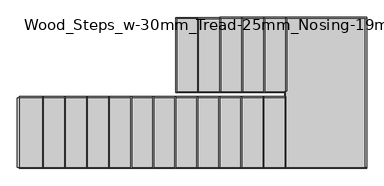
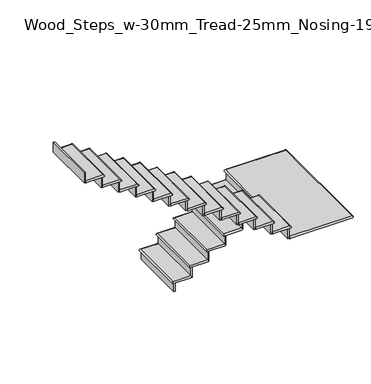
"""IFC4 building model written with IfcOpenShell, lengths in millimetres: stair flight geometry, Wood_Steps_w-30mm_Tread-25mm_Nosing-19mm_Riser."""

from ifc_helpers import new_model, si_unit, frame, origin, place, context, project, spatial, circle_curve, ellipse_curve, faceted_brep, source, transform, mapped, element, save
from ifc_brep_helpers import plane_surface, cylinder_surface, advanced_brep


def wood_steps_w_30mm_tread_25mm_nosing_19mm_riser_5243a390(model_context):
    return source(origin(), model_context, "Body", "SolidModel", [
        advanced_brep(
        [(-8665.149573, -11058.3255223, 782.8), (-8665.149573, -11058.3255223, 812.8), (-8665.149573, -10219.6521308, 812.8), (-8665.149573, -10219.6521308, 782.8), (-8400.9545789, -11058.3255223, 812.8), (-8400.9545789, -10219.6521308, 812.8), (-8400.9545789, -10219.6521308, 782.8), (-8400.9545789, -11058.3255223, 782.8)],
        [
            (0, 1, ellipse_curve(frame((-8665.149573, -11058.3255223, 797.8), z_axis=(-0.707106781186546, 0.707106781186549, 0.0), x_axis=(-0.707106781186549, -0.7071067811865461, 0.0)), 21.2132034, 15.0)),
            (1, 2),
            (2, 3, ellipse_curve(frame((-8665.149573, -10219.6521308, 797.8), z_axis=(-0.7071067811865489, -0.7071067811865461, 0.0), x_axis=(0.7071067811865462, -0.7071067811865489, 0.0)), 21.2132034, 15.0)),
            (3, 0),
            (4, 5),
            (5, 2),
            (1, 4),
            (6, 7),
            (7, 0),
            (3, 6),
            (4, 7, circle_curve(frame((-8400.9545789, -11058.3255223, 797.8), z_axis=(1.0, 0.0, 0.0), x_axis=(0.0, 1.0, 0.0)), 15.0)),
            (6, 5, circle_curve(frame((-8400.9545789, -10219.6521308, 797.8), z_axis=(1.0, 0.0, 0.0), x_axis=(0.0, -1.0, 0.0)), 15.0)),
        ],
        [
            cylinder_surface(frame((-8665.149573, -11058.3255223, 797.8), z_axis=(0.0, -1.0, 0.0), x_axis=(1.0, 0.0, 0.0)), 15.0),
            plane_surface(frame((-6495.4132565, -10219.6521308, 812.8), z_axis=(0.0, 0.0, 1.0), x_axis=(-1.0, 0.0, 0.0))),
            plane_surface(frame((-6495.4132565, -10219.6521308, 782.8), z_axis=(0.0, 0.0, -1.0), x_axis=(1.0, 0.0, 0.0))),
            plane_surface(frame((-8400.9545789, -11058.3255223, 812.8), z_axis=(1.0, 0.0, 0.0), x_axis=(0.0, 0.0, -1.0))),
            cylinder_surface(frame((-8400.9545789, -11058.3255223, 797.8), z_axis=(1.0, 0.0, 0.0), x_axis=(0.0, 1.0, 0.0)), 15.0),
            cylinder_surface(frame((-8665.149573, -10219.6521308, 797.8), z_axis=(-1.0, 0.0, 0.0), x_axis=(0.0, -1.0, 0.0)), 15.0),
        ],
        [
            (0, [[1, 2, 3, 4]]),
            (1, [[5, 6, -2, 7]]),
            (2, [[8, 9, -4, 10]]),
            (3, [[-5, 11, -8, 12]]),
            (4, [[-11, -7, -1, -9]]),
            (5, [[-3, -6, -12, -10]]),
        ],
    ),
        faceted_brep([(-8655.149573, -11058.3255223, 782.8), (-8655.149573, -11058.3255223, 650.24), (-8636.149573, -11058.3255223, 650.24), (-8636.149573, -11058.3255223, 782.8), (-8655.149573, -10219.6521308, 782.8), (-8636.149573, -10219.6521308, 782.8), (-8636.149573, -10219.6521308, 650.24), (-8655.149573, -10219.6521308, 650.24)], [[[0, 1, 2, 3]], [[4, 5, 6, 7]], [[1, 0, 4, 7]], [[2, 1, 7, 6]], [[3, 2, 6, 5]], [[0, 3, 5, 4]]]),
        faceted_brep([(-8400.9545789, -11058.3255223, 945.36), (-8400.9545789, -11058.3255223, 782.8), (-8381.9545789, -11058.3255223, 782.8), (-8381.9545789, -11058.3255223, 945.36), (-8400.9545789, -10219.6521308, 945.36), (-8381.9545789, -10219.6521308, 945.36), (-8381.9545789, -10219.6521308, 782.8), (-8400.9545789, -10219.6521308, 782.8)], [[[0, 1, 2, 3]], [[4, 5, 6, 7]], [[1, 0, 4, 7]], [[2, 1, 7, 6]], [[3, 2, 6, 5]], [[0, 3, 5, 4]]]),
        advanced_brep(
        [(-8146.7595849, -11058.3255223, 975.36), (-8146.7595849, -10219.6521308, 975.36), (-8410.9545789, -10219.6521308, 975.36), (-8410.9545789, -11058.3255223, 975.36), (-8146.7595849, -10219.6521308, 945.36), (-8146.7595849, -11058.3255223, 945.36), (-8410.9545789, -11058.3255223, 945.36), (-8410.9545789, -10219.6521308, 945.36)],
        [
            (0, 1),
            (1, 2),
            (2, 3),
            (3, 0),
            (4, 5),
            (5, 6),
            (6, 7),
            (7, 4),
            (0, 5, circle_curve(frame((-8146.7595849, -11058.3255223, 960.36), z_axis=(1.0, 0.0, 0.0), x_axis=(0.0, 1.0, 0.0)), 15.0)),
            (4, 1, circle_curve(frame((-8146.7595849, -10219.6521308, 960.36), z_axis=(1.0, 0.0, 0.0), x_axis=(0.0, -1.0, 0.0)), 15.0)),
            (6, 3, ellipse_curve(frame((-8410.9545789, -11058.3255223, 960.36), z_axis=(-0.707106781186546, 0.707106781186549, 0.0), x_axis=(-0.707106781186549, -0.7071067811865461, 0.0)), 21.2132034, 15.0)),
            (2, 7, ellipse_curve(frame((-8410.9545789, -10219.6521308, 960.36), z_axis=(-0.7071067811865489, -0.7071067811865461, 0.0), x_axis=(0.7071067811865462, -0.7071067811865489, 0.0)), 21.2132034, 15.0)),
        ],
        [
            plane_surface(frame((-6495.4132565, -10219.6521308, 975.36), z_axis=(0.0, 0.0, 1.0), x_axis=(-1.0, 0.0, 0.0))),
            plane_surface(frame((-6495.4132565, -10219.6521308, 945.36), z_axis=(0.0, 0.0, -1.0), x_axis=(1.0, 0.0, 0.0))),
            plane_surface(frame((-8146.7595849, -11058.3255223, 975.36), z_axis=(1.0, 0.0, 0.0), x_axis=(0.0, 0.0, -1.0))),
            cylinder_surface(frame((-8410.9545789, -11058.3255223, 960.36), z_axis=(0.0, -1.0, 0.0), x_axis=(1.0, 0.0, 0.0)), 15.0),
            cylinder_surface(frame((-8146.7595849, -11058.3255223, 960.36), z_axis=(1.0, 0.0, 0.0), x_axis=(0.0, 1.0, 0.0)), 15.0),
            cylinder_surface(frame((-8410.9545789, -10219.6521308, 960.36), z_axis=(-1.0, 0.0, 0.0), x_axis=(0.0, -1.0, 0.0)), 15.0),
        ],
        [
            (0, [[1, 2, 3, 4]]),
            (1, [[5, 6, 7, 8]]),
            (2, [[-1, 9, -5, 10]]),
            (3, [[11, -3, 12, -7]]),
            (4, [[-9, -4, -11, -6]]),
            (5, [[-12, -2, -10, -8]]),
        ],
    ),
        faceted_brep([(-8146.7595849, -11058.3255223, 1107.92), (-8146.7595849, -11058.3255223, 945.36), (-8127.7595849, -11058.3255223, 945.36), (-8127.7595849, -11058.3255223, 1107.92), (-8146.7595849, -10219.6521308, 1107.92), (-8127.7595849, -10219.6521308, 1107.92), (-8127.7595849, -10219.6521308, 945.36), (-8146.7595849, -10219.6521308, 945.36)], [[[0, 1, 2, 3]], [[4, 5, 6, 7]], [[1, 0, 4, 7]], [[2, 1, 7, 6]], [[3, 2, 6, 5]], [[0, 3, 5, 4]]]),
        advanced_brep(
        [(-7893.1206135, -11058.3255223, 1137.92), (-7893.1206135, -10219.6521308, 1137.92), (-8156.7595849, -10219.6521308, 1137.92), (-8156.7595849, -11058.3255223, 1137.92), (-7893.1206135, -10219.6521308, 1107.92), (-7893.1206135, -11058.3255223, 1107.92), (-8156.7595849, -11058.3255223, 1107.92), (-8156.7595849, -10219.6521308, 1107.92)],
        [
            (0, 1),
            (1, 2),
            (2, 3),
            (3, 0),
            (4, 5),
            (5, 6),
            (6, 7),
            (7, 4),
            (0, 5, circle_curve(frame((-7893.1206135, -11058.3255223, 1122.92), z_axis=(1.0, 0.0, 0.0), x_axis=(0.0, 1.0, 0.0)), 15.0)),
            (4, 1, circle_curve(frame((-7893.1206135, -10219.6521308, 1122.92), z_axis=(1.0, 0.0, 0.0), x_axis=(0.0, -1.0, 0.0)), 15.0)),
            (6, 3, ellipse_curve(frame((-8156.7595849, -11058.3255223, 1122.92), z_axis=(-0.707106781186546, 0.707106781186549, 0.0), x_axis=(-0.707106781186549, -0.7071067811865461, 0.0)), 21.2132034, 15.0)),
            (2, 7, ellipse_curve(frame((-8156.7595849, -10219.6521308, 1122.92), z_axis=(-0.7071067811865489, -0.7071067811865461, 0.0), x_axis=(0.7071067811865462, -0.7071067811865489, 0.0)), 21.2132034, 15.0)),
        ],
        [
            plane_surface(frame((-6495.4132565, -10219.6521308, 1137.92), z_axis=(0.0, 0.0, 1.0), x_axis=(-1.0, 0.0, 0.0))),
            plane_surface(frame((-6495.4132565, -10219.6521308, 1107.92), z_axis=(0.0, 0.0, -1.0), x_axis=(1.0, 0.0, 0.0))),
            plane_surface(frame((-7893.1206135, -11058.3255223, 1137.92), z_axis=(1.0, 0.0, 0.0), x_axis=(0.0, 0.0, -1.0))),
            cylinder_surface(frame((-8156.7595849, -11058.3255223, 1122.92), z_axis=(0.0, -1.0, 0.0), x_axis=(1.0, 0.0, 0.0)), 15.0),
            cylinder_surface(frame((-7893.1206135, -11058.3255223, 1122.92), z_axis=(1.0, 0.0, 0.0), x_axis=(0.0, 1.0, 0.0)), 15.0),
            cylinder_surface(frame((-8156.7595849, -10219.6521308, 1122.92), z_axis=(-1.0, 0.0, 0.0), x_axis=(0.0, -1.0, 0.0)), 15.0),
        ],
        [
            (0, [[1, 2, 3, 4]]),
            (1, [[5, 6, 7, 8]]),
            (2, [[-1, 9, -5, 10]]),
            (3, [[11, -3, 12, -7]]),
            (4, [[-9, -4, -11, -6]]),
            (5, [[-12, -2, -10, -8]]),
        ],
    ),
        faceted_brep([(-7893.1206135, -11058.3255223, 1270.48), (-7893.1206135, -11058.3255223, 1107.92), (-7874.1206135, -11058.3255223, 1107.92), (-7874.1206135, -11058.3255223, 1270.48), (-7893.1206135, -10219.6521308, 1270.48), (-7874.1206135, -10219.6521308, 1270.48), (-7874.1206135, -10219.6521308, 1107.92), (-7893.1206135, -10219.6521308, 1107.92)], [[[0, 1, 2, 3]], [[4, 5, 6, 7]], [[1, 0, 4, 7]], [[2, 1, 7, 6]], [[3, 2, 6, 5]], [[0, 3, 5, 4]]]),
        advanced_brep(
        [(-7638.9256194, -11058.3255223, 1300.48), (-7638.9256194, -10219.6521308, 1300.48), (-7903.1206135, -10219.6521308, 1300.48), (-7903.1206135, -11058.3255223, 1300.48), (-7638.9256194, -10219.6521308, 1270.48), (-7638.9256194, -11058.3255223, 1270.48), (-7903.1206135, -11058.3255223, 1270.48), (-7903.1206135, -10219.6521308, 1270.48)],
        [
            (0, 1),
            (1, 2),
            (2, 3),
            (3, 0),
            (4, 5),
            (5, 6),
            (6, 7),
            (7, 4),
            (0, 5, circle_curve(frame((-7638.9256194, -11058.3255223, 1285.48), z_axis=(1.0, 0.0, 0.0), x_axis=(0.0, 1.0, 0.0)), 15.0)),
            (4, 1, circle_curve(frame((-7638.9256194, -10219.6521308, 1285.48), z_axis=(1.0, 0.0, 0.0), x_axis=(0.0, -1.0, 0.0)), 15.0)),
            (6, 3, ellipse_curve(frame((-7903.1206135, -11058.3255223, 1285.48), z_axis=(-0.707106781186546, 0.707106781186549, 0.0), x_axis=(-0.707106781186549, -0.7071067811865461, 0.0)), 21.2132034, 15.0)),
            (2, 7, ellipse_curve(frame((-7903.1206135, -10219.6521308, 1285.48), z_axis=(-0.7071067811865489, -0.7071067811865461, 0.0), x_axis=(0.7071067811865462, -0.7071067811865489, 0.0)), 21.2132034, 15.0)),
        ],
        [
            plane_surface(frame((-6495.4132565, -10219.6521308, 1300.48), z_axis=(0.0, 0.0, 1.0), x_axis=(-1.0, 0.0, 0.0))),
            plane_surface(frame((-6495.4132565, -10219.6521308, 1270.48), z_axis=(0.0, 0.0, -1.0), x_axis=(1.0, 0.0, 0.0))),
            plane_surface(frame((-7638.9256194, -11058.3255223, 1300.48), z_axis=(1.0, 0.0, 0.0), x_axis=(0.0, 0.0, -1.0))),
            cylinder_surface(frame((-7903.1206135, -11058.3255223, 1285.48), z_axis=(0.0, -1.0, 0.0), x_axis=(1.0, 0.0, 0.0)), 15.0),
            cylinder_surface(frame((-7638.9256194, -11058.3255223, 1285.48), z_axis=(1.0, 0.0, 0.0), x_axis=(0.0, 1.0, 0.0)), 15.0),
            cylinder_surface(frame((-7903.1206135, -10219.6521308, 1285.48), z_axis=(-1.0, 0.0, 0.0), x_axis=(0.0, -1.0, 0.0)), 15.0),
        ],
        [
            (0, [[1, 2, 3, 4]]),
            (1, [[5, 6, 7, 8]]),
            (2, [[-1, 9, -5, 10]]),
            (3, [[11, -3, 12, -7]]),
            (4, [[-9, -4, -11, -6]]),
            (5, [[-12, -2, -10, -8]]),
        ],
    ),
        faceted_brep([(-7384.7306254, -11058.3255223, 1595.6), (-7384.7306254, -11058.3255223, 1433.04), (-7365.7306254, -11058.3255223, 1433.04), (-7365.7306254, -11058.3255223, 1595.6), (-7384.7306254, -10219.6521308, 1595.6), (-7365.7306254, -10219.6521308, 1595.6), (-7365.7306254, -10219.6521308, 1433.04), (-7384.7306254, -10219.6521308, 1433.04)], [[[0, 1, 2, 3]], [[4, 5, 6, 7]], [[1, 0, 4, 7]], [[2, 1, 7, 6]], [[3, 2, 6, 5]], [[0, 3, 5, 4]]]),
        faceted_brep([(-7434.7306254, -11134.5255223, 1758.16), (-7434.7306254, -11134.5255223, 1595.6), (-7453.7306254, -11134.5255223, 1595.6), (-7453.7306254, -11134.5255223, 1758.16), (-7434.7306254, -11934.0860066, 1758.16), (-7453.7306254, -11934.0860066, 1758.16), (-7453.7306254, -11934.0860066, 1595.6), (-7434.7306254, -11934.0860066, 1595.6)], [[[0, 1, 2, 3]], [[4, 5, 6, 7]], [[1, 0, 4, 7]], [[2, 1, 7, 6]], [[3, 2, 6, 5]], [[0, 3, 5, 4]]]),
        advanced_brep(
        [(-7688.9256194, -11134.5255223, 1788.16), (-7688.9256194, -11934.0860066, 1788.16), (-7424.7306254, -11934.0860066, 1788.16), (-7424.7306254, -11134.5255223, 1788.16), (-7688.9256194, -11934.0860066, 1758.16), (-7688.9256194, -11134.5255223, 1758.16), (-7424.7306254, -11134.5255223, 1758.16), (-7424.7306254, -11934.0860066, 1758.16)],
        [
            (0, 1),
            (1, 2),
            (2, 3),
            (3, 0),
            (4, 5),
            (5, 6),
            (6, 7),
            (7, 4),
            (0, 5, circle_curve(frame((-7688.9256194, -11134.5255223, 1773.16), z_axis=(-1.0, 0.0, 0.0), x_axis=(0.0, -1.0, 0.0)), 15.0)),
            (4, 1, circle_curve(frame((-7688.9256194, -11934.0860066, 1773.16), z_axis=(-1.0, 0.0, 0.0), x_axis=(0.0, 1.0, 0.0)), 15.0)),
            (6, 3, ellipse_curve(frame((-7424.7306254, -11134.5255223, 1773.16), z_axis=(0.7071067811865458, -0.7071067811865492, 0.0), x_axis=(0.7071067811865493, 0.7071067811865457, 0.0)), 21.2132034, 15.0)),
            (2, 7, ellipse_curve(frame((-7424.7306254, -11934.0860066, 1773.16), z_axis=(0.7071067811865491, 0.7071067811865459, 0.0), x_axis=(-0.7071067811865459, 0.7071067811865491, 0.0)), 21.2132034, 15.0)),
        ],
        [
            plane_surface(frame((-10457.8773536, -11934.0860066, 1788.16), z_axis=(0.0, 0.0, 1.0), x_axis=(1.0, 0.0, 0.0))),
            plane_surface(frame((-10457.8773536, -11934.0860066, 1758.16), z_axis=(0.0, 0.0, -1.0), x_axis=(-1.0, 0.0, 0.0))),
            plane_surface(frame((-7688.9256194, -11134.5255223, 1788.16), z_axis=(-1.0, 0.0, 0.0), x_axis=(0.0, 0.0, -1.0))),
            cylinder_surface(frame((-7424.7306254, -11134.5255223, 1773.16), z_axis=(0.0, 1.0, 0.0), x_axis=(-1.0, 0.0, 0.0)), 15.0),
            cylinder_surface(frame((-7688.9256194, -11134.5255223, 1773.16), z_axis=(-1.0, 0.0, 0.0), x_axis=(0.0, -1.0, 0.0)), 15.0),
            cylinder_surface(frame((-7424.7306254, -11934.0860066, 1773.16), z_axis=(1.0, 0.0, 0.0), x_axis=(0.0, 1.0, 0.0)), 15.0),
        ],
        [
            (0, [[1, 2, 3, 4]]),
            (1, [[5, 6, 7, 8]]),
            (2, [[-1, 9, -5, 10]]),
            (3, [[11, -3, 12, -7]]),
            (4, [[-9, -4, -11, -6]]),
            (5, [[-12, -2, -10, -8]]),
        ],
    ),
        faceted_brep([(-8196.7595849, -11134.5255223, 2245.84), (-8196.7595849, -11134.5255223, 2083.28), (-8215.7595849, -11134.5255223, 2083.28), (-8215.7595849, -11134.5255223, 2245.84), (-8196.7595849, -11934.0860066, 2245.84), (-8215.7595849, -11934.0860066, 2245.84), (-8215.7595849, -11934.0860066, 2083.28), (-8196.7595849, -11934.0860066, 2083.28)], [[[0, 1, 2, 3]], [[4, 5, 6, 7]], [[1, 0, 4, 7]], [[2, 1, 7, 6]], [[3, 2, 6, 5]], [[0, 3, 5, 4]]]),
        advanced_brep(
        [(-8450.9545789, -11134.5255223, 2275.84), (-8450.9545789, -11934.0860066, 2275.84), (-8186.7595849, -11934.0860066, 2275.84), (-8186.7595849, -11134.5255223, 2275.84), (-8450.9545789, -11934.0860066, 2245.84), (-8450.9545789, -11134.5255223, 2245.84), (-8186.7595849, -11134.5255223, 2245.84), (-8186.7595849, -11934.0860066, 2245.84)],
        [
            (0, 1),
            (1, 2),
            (2, 3),
            (3, 0),
            (4, 5),
            (5, 6),
            (6, 7),
            (7, 4),
            (0, 5, circle_curve(frame((-8450.9545789, -11134.5255223, 2260.84), z_axis=(-1.0, 0.0, 0.0), x_axis=(0.0, -1.0, 0.0)), 15.0)),
            (4, 1, circle_curve(frame((-8450.9545789, -11934.0860066, 2260.84), z_axis=(-1.0, 0.0, 0.0), x_axis=(0.0, 1.0, 0.0)), 15.0)),
            (6, 3, ellipse_curve(frame((-8186.7595849, -11134.5255223, 2260.84), z_axis=(0.7071067811865458, -0.7071067811865492, 0.0), x_axis=(0.7071067811865493, 0.7071067811865457, 0.0)), 21.2132034, 15.0)),
            (2, 7, ellipse_curve(frame((-8186.7595849, -11934.0860066, 2260.84), z_axis=(0.7071067811865491, 0.7071067811865459, 0.0), x_axis=(-0.7071067811865459, 0.7071067811865491, 0.0)), 21.2132034, 15.0)),
        ],
        [
            plane_surface(frame((-10457.8773536, -11934.0860066, 2275.84), z_axis=(0.0, 0.0, 1.0), x_axis=(1.0, 0.0, 0.0))),
            plane_surface(frame((-10457.8773536, -11934.0860066, 2245.84), z_axis=(0.0, 0.0, -1.0), x_axis=(-1.0, 0.0, 0.0))),
            plane_surface(frame((-8450.9545789, -11134.5255223, 2275.84), z_axis=(-1.0, 0.0, 0.0), x_axis=(0.0, 0.0, -1.0))),
            cylinder_surface(frame((-8186.7595849, -11134.5255223, 2260.84), z_axis=(0.0, 1.0, 0.0), x_axis=(-1.0, 0.0, 0.0)), 15.0),
            cylinder_surface(frame((-8450.9545789, -11134.5255223, 2260.84), z_axis=(-1.0, 0.0, 0.0), x_axis=(0.0, -1.0, 0.0)), 15.0),
            cylinder_surface(frame((-8186.7595849, -11934.0860066, 2260.84), z_axis=(1.0, 0.0, 0.0), x_axis=(0.0, 1.0, 0.0)), 15.0),
        ],
        [
            (0, [[1, 2, 3, 4]]),
            (1, [[5, 6, 7, 8]]),
            (2, [[-1, 9, -5, 10]]),
            (3, [[11, -3, 12, -7]]),
            (4, [[-9, -4, -11, -6]]),
            (5, [[-12, -2, -10, -8]]),
        ],
    ),
        faceted_brep([(-8958.7885444, -11134.5255223, 2733.52), (-8958.7885444, -11134.5255223, 2570.96), (-8977.7885444, -11134.5255223, 2570.96), (-8977.7885444, -11134.5255223, 2733.52), (-8958.7885444, -11934.0860066, 2733.52), (-8977.7885444, -11934.0860066, 2733.52), (-8977.7885444, -11934.0860066, 2570.96), (-8958.7885444, -11934.0860066, 2570.96)], [[[0, 1, 2, 3]], [[4, 5, 6, 7]], [[1, 0, 4, 7]], [[2, 1, 7, 6]], [[3, 2, 6, 5]], [[0, 3, 5, 4]]]),
        advanced_brep(
        [(-9212.9835384, -11134.5255223, 2763.52), (-9212.9835384, -11934.0860066, 2763.52), (-8948.7885444, -11934.0860066, 2763.52), (-8948.7885444, -11134.5255223, 2763.52), (-9212.9835384, -11934.0860066, 2733.52), (-9212.9835384, -11134.5255223, 2733.52), (-8948.7885444, -11134.5255223, 2733.52), (-8948.7885444, -11934.0860066, 2733.52)],
        [
            (0, 1),
            (1, 2),
            (2, 3),
            (3, 0),
            (4, 5),
            (5, 6),
            (6, 7),
            (7, 4),
            (0, 5, circle_curve(frame((-9212.9835384, -11134.5255223, 2748.52), z_axis=(-1.0, 0.0, 0.0), x_axis=(0.0, -1.0, 0.0)), 15.0)),
            (4, 1, circle_curve(frame((-9212.9835384, -11934.0860066, 2748.52), z_axis=(-1.0, 0.0, 0.0), x_axis=(0.0, 1.0, 0.0)), 15.0)),
            (6, 3, ellipse_curve(frame((-8948.7885444, -11134.5255223, 2748.52), z_axis=(0.7071067811865458, -0.7071067811865492, 0.0), x_axis=(0.7071067811865493, 0.7071067811865457, 0.0)), 21.2132034, 15.0)),
            (2, 7, ellipse_curve(frame((-8948.7885444, -11934.0860066, 2748.52), z_axis=(0.7071067811865491, 0.7071067811865459, 0.0), x_axis=(-0.7071067811865459, 0.7071067811865491, 0.0)), 21.2132034, 15.0)),
        ],
        [
            plane_surface(frame((-10457.8773536, -11934.0860066, 2763.52), z_axis=(0.0, 0.0, 1.0), x_axis=(1.0, 0.0, 0.0))),
            plane_surface(frame((-10457.8773536, -11934.0860066, 2733.52), z_axis=(0.0, 0.0, -1.0), x_axis=(-1.0, 0.0, 0.0))),
            plane_surface(frame((-9212.9835384, -11134.5255223, 2763.52), z_axis=(-1.0, 0.0, 0.0), x_axis=(0.0, 0.0, -1.0))),
            cylinder_surface(frame((-8948.7885444, -11134.5255223, 2748.52), z_axis=(0.0, 1.0, 0.0), x_axis=(-1.0, 0.0, 0.0)), 15.0),
            cylinder_surface(frame((-9212.9835384, -11134.5255223, 2748.52), z_axis=(-1.0, 0.0, 0.0), x_axis=(0.0, -1.0, 0.0)), 15.0),
            cylinder_surface(frame((-8948.7885444, -11934.0860066, 2748.52), z_axis=(1.0, 0.0, 0.0), x_axis=(0.0, 1.0, 0.0)), 15.0),
        ],
        [
            (0, [[1, 2, 3, 4]]),
            (1, [[5, 6, 7, 8]]),
            (2, [[-1, 9, -5, 10]]),
            (3, [[11, -3, 12, -7]]),
            (4, [[-9, -4, -11, -6]]),
            (5, [[-12, -2, -10, -8]]),
        ],
    ),
        faceted_brep([(-9212.9835384, -11134.5255223, 2896.08), (-9212.9835384, -11134.5255223, 2733.52), (-9231.9835384, -11134.5255223, 2733.52), (-9231.9835384, -11134.5255223, 2896.08), (-9212.9835384, -11934.0860066, 2896.08), (-9231.9835384, -11934.0860066, 2896.08), (-9231.9835384, -11934.0860066, 2733.52), (-9212.9835384, -11934.0860066, 2733.52)], [[[0, 1, 2, 3]], [[4, 5, 6, 7]], [[1, 0, 4, 7]], [[2, 1, 7, 6]], [[3, 2, 6, 5]], [[0, 3, 5, 4]]]),
        advanced_brep(
        [(-9466.6534, -11134.5255223, 2926.08), (-9466.6534, -11934.0860066, 2926.08), (-9202.9835384, -11934.0860066, 2926.08), (-9202.9835384, -11134.5255223, 2926.08), (-9466.6534, -11934.0860066, 2896.08), (-9466.6534, -11134.5255223, 2896.08), (-9202.9835384, -11134.5255223, 2896.08), (-9202.9835384, -11934.0860066, 2896.08)],
        [
            (0, 1),
            (1, 2),
            (2, 3),
            (3, 0),
            (4, 5),
            (5, 6),
            (6, 7),
            (7, 4),
            (0, 5, circle_curve(frame((-9466.6534, -11134.5255223, 2911.08), z_axis=(-1.0, 0.0, 0.0), x_axis=(0.0, -1.0, 0.0)), 15.0)),
            (4, 1, circle_curve(frame((-9466.6534, -11934.0860066, 2911.08), z_axis=(-1.0, 0.0, 0.0), x_axis=(0.0, 1.0, 0.0)), 15.0)),
            (6, 3, ellipse_curve(frame((-9202.9835384, -11134.5255223, 2911.08), z_axis=(0.7071067811865458, -0.7071067811865492, 0.0), x_axis=(0.7071067811865493, 0.7071067811865457, 0.0)), 21.2132034, 15.0)),
            (2, 7, ellipse_curve(frame((-9202.9835384, -11934.0860066, 2911.08), z_axis=(0.7071067811865491, 0.7071067811865459, 0.0), x_axis=(-0.7071067811865459, 0.7071067811865491, 0.0)), 21.2132034, 15.0)),
        ],
        [
            plane_surface(frame((-10457.8773536, -11934.0860066, 2926.08), z_axis=(0.0, 0.0, 1.0), x_axis=(1.0, 0.0, 0.0))),
            plane_surface(frame((-10457.8773536, -11934.0860066, 2896.08), z_axis=(0.0, 0.0, -1.0), x_axis=(-1.0, 0.0, 0.0))),
            plane_surface(frame((-9466.6534, -11134.5255223, 2926.08), z_axis=(-1.0, 0.0, 0.0), x_axis=(0.0, 0.0, -1.0))),
            cylinder_surface(frame((-9202.9835384, -11134.5255223, 2911.08), z_axis=(0.0, 1.0, 0.0), x_axis=(-1.0, 0.0, 0.0)), 15.0),
            cylinder_surface(frame((-9466.6534, -11134.5255223, 2911.08), z_axis=(-1.0, 0.0, 0.0), x_axis=(0.0, -1.0, 0.0)), 15.0),
            cylinder_surface(frame((-9202.9835384, -11934.0860066, 2911.08), z_axis=(1.0, 0.0, 0.0), x_axis=(0.0, 1.0, 0.0)), 15.0),
        ],
        [
            (0, [[1, 2, 3, 4]]),
            (1, [[5, 6, 7, 8]]),
            (2, [[-1, 9, -5, 10]]),
            (3, [[11, -3, 12, -7]]),
            (4, [[-9, -4, -11, -6]]),
            (5, [[-12, -2, -10, -8]]),
        ],
    ),
        faceted_brep([(-9720.8175039, -11134.5255223, 3221.2), (-9720.8175039, -11134.5255223, 3058.64), (-9739.8175039, -11134.5255223, 3058.64), (-9739.8175039, -11134.5255223, 3221.2), (-9720.8175039, -11934.0860066, 3221.2), (-9739.8175039, -11934.0860066, 3221.2), (-9739.8175039, -11934.0860066, 3058.64), (-9720.8175039, -11934.0860066, 3058.64)], [[[0, 1, 2, 3]], [[4, 5, 6, 7]], [[1, 0, 4, 7]], [[2, 1, 7, 6]], [[3, 2, 6, 5]], [[0, 3, 5, 4]]]),
        advanced_brep(
        [(-9975.012498, -11134.5255223, 3251.2), (-9975.012498, -11934.0860066, 3251.2), (-9710.8175039, -11934.0860066, 3251.2), (-9710.8175039, -11134.5255223, 3251.2), (-9975.012498, -11934.0860066, 3221.2), (-9975.012498, -11134.5255223, 3221.2), (-9710.8175039, -11134.5255223, 3221.2), (-9710.8175039, -11934.0860066, 3221.2)],
        [
            (0, 1),
            (1, 2),
            (2, 3),
            (3, 0),
            (4, 5),
            (5, 6),
            (6, 7),
            (7, 4),
            (0, 5, circle_curve(frame((-9975.012498, -11134.5255223, 3236.2), z_axis=(-1.0, 0.0, 0.0), x_axis=(0.0, -1.0, 0.0)), 15.0)),
            (4, 1, circle_curve(frame((-9975.012498, -11934.0860066, 3236.2), z_axis=(-1.0, 0.0, 0.0), x_axis=(0.0, 1.0, 0.0)), 15.0)),
            (6, 3, ellipse_curve(frame((-9710.8175039, -11134.5255223, 3236.2), z_axis=(0.7071067811865458, -0.7071067811865492, 0.0), x_axis=(0.7071067811865493, 0.7071067811865457, 0.0)), 21.2132034, 15.0)),
            (2, 7, ellipse_curve(frame((-9710.8175039, -11934.0860066, 3236.2), z_axis=(0.7071067811865491, 0.7071067811865459, 0.0), x_axis=(-0.7071067811865459, 0.7071067811865491, 0.0)), 21.2132034, 15.0)),
        ],
        [
            plane_surface(frame((-10457.8773536, -11934.0860066, 3251.2), z_axis=(0.0, 0.0, 1.0), x_axis=(1.0, 0.0, 0.0))),
            plane_surface(frame((-10457.8773536, -11934.0860066, 3221.2), z_axis=(0.0, 0.0, -1.0), x_axis=(-1.0, 0.0, 0.0))),
            plane_surface(frame((-9975.012498, -11134.5255223, 3251.2), z_axis=(-1.0, 0.0, 0.0), x_axis=(0.0, 0.0, -1.0))),
            cylinder_surface(frame((-9710.8175039, -11134.5255223, 3236.2), z_axis=(0.0, 1.0, 0.0), x_axis=(-1.0, 0.0, 0.0)), 15.0),
            cylinder_surface(frame((-9975.012498, -11134.5255223, 3236.2), z_axis=(-1.0, 0.0, 0.0), x_axis=(0.0, -1.0, 0.0)), 15.0),
            cylinder_surface(frame((-9710.8175039, -11934.0860066, 3236.2), z_axis=(1.0, 0.0, 0.0), x_axis=(0.0, 1.0, 0.0)), 15.0),
        ],
        [
            (0, [[1, 2, 3, 4]]),
            (1, [[5, 6, 7, 8]]),
            (2, [[-1, 9, -5, 10]]),
            (3, [[11, -3, 12, -7]]),
            (4, [[-9, -4, -11, -6]]),
            (5, [[-12, -2, -10, -8]]),
        ],
    ),
        faceted_brep([(-9975.012498, -11134.5255223, 3383.76), (-9975.012498, -11134.5255223, 3221.2), (-9994.012498, -11134.5255223, 3221.2), (-9994.012498, -11134.5255223, 3383.76), (-9975.012498, -11934.0860066, 3383.76), (-9994.012498, -11934.0860066, 3383.76), (-9994.012498, -11934.0860066, 3221.2), (-9975.012498, -11934.0860066, 3221.2)], [[[0, 1, 2, 3]], [[4, 5, 6, 7]], [[1, 0, 4, 7]], [[2, 1, 7, 6]], [[3, 2, 6, 5]], [[0, 3, 5, 4]]]),
        advanced_brep(
        [(-10228.6823595, -11134.5255223, 3413.76), (-10228.6823595, -11934.0860066, 3413.76), (-9965.012498, -11934.0860066, 3413.76), (-9965.012498, -11134.5255223, 3413.76), (-10228.6823595, -11934.0860066, 3383.76), (-10228.6823595, -11134.5255223, 3383.76), (-9965.012498, -11134.5255223, 3383.76), (-9965.012498, -11934.0860066, 3383.76)],
        [
            (0, 1),
            (1, 2),
            (2, 3),
            (3, 0),
            (4, 5),
            (5, 6),
            (6, 7),
            (7, 4),
            (0, 5, circle_curve(frame((-10228.6823595, -11134.5255223, 3398.76), z_axis=(-1.0, 0.0, 0.0), x_axis=(0.0, -1.0, 0.0)), 15.0)),
            (4, 1, circle_curve(frame((-10228.6823595, -11934.0860066, 3398.76), z_axis=(-1.0, 0.0, 0.0), x_axis=(0.0, 1.0, 0.0)), 15.0)),
            (6, 3, ellipse_curve(frame((-9965.012498, -11134.5255223, 3398.76), z_axis=(0.7071067811865454, -0.7071067811865498, 0.0), x_axis=(0.7071067811865498, 0.7071067811865451, 0.0)), 21.2132034, 15.0)),
            (2, 7, ellipse_curve(frame((-9965.012498, -11934.0860066, 3398.76), z_axis=(0.7071067811865496, 0.7071067811865454, 0.0), x_axis=(-0.7071067811865452, 0.7071067811865498, 0.0)), 21.2132034, 15.0)),
        ],
        [
            plane_surface(frame((-10457.8773536, -11934.0860066, 3413.76), z_axis=(0.0, 0.0, 1.0), x_axis=(1.0, 0.0, 0.0))),
            plane_surface(frame((-10457.8773536, -11934.0860066, 3383.76), z_axis=(0.0, 0.0, -1.0), x_axis=(-1.0, 0.0, 0.0))),
            plane_surface(frame((-10228.6823595, -11134.5255223, 3413.76), z_axis=(-1.0, 0.0, 0.0), x_axis=(0.0, 0.0, -1.0))),
            cylinder_surface(frame((-9965.012498, -11134.5255223, 3398.76), z_axis=(0.0, 1.0, 0.0), x_axis=(-1.0, 0.0, 0.0)), 15.0),
            cylinder_surface(frame((-10228.6823595, -11134.5255223, 3398.76), z_axis=(-1.0, 0.0, 0.0), x_axis=(0.0, -1.0, 0.0)), 15.0),
            cylinder_surface(frame((-9965.012498, -11934.0860066, 3398.76), z_axis=(1.0, 0.0, 0.0), x_axis=(0.0, 1.0, 0.0)), 15.0),
        ],
        [
            (0, [[1, 2, 3, 4]]),
            (1, [[5, 6, 7, 8]]),
            (2, [[-1, 9, -5, 10]]),
            (3, [[11, -3, 12, -7]]),
            (4, [[-9, -4, -11, -6]]),
            (5, [[-12, -2, -10, -8]]),
        ],
    ),
        faceted_brep([(-10482.8773536, -11134.5255223, 3708.88), (-10482.8773536, -11134.5255223, 3546.32), (-10501.8773536, -11134.5255223, 3546.32), (-10501.8773536, -11134.5255223, 3708.88), (-10482.8773536, -11934.0860066, 3708.88), (-10501.8773536, -11934.0860066, 3708.88), (-10501.8773536, -11934.0860066, 3546.32), (-10482.8773536, -11934.0860066, 3546.32)], [[[0, 1, 2, 3]], [[4, 5, 6, 7]], [[1, 0, 4, 7]], [[2, 1, 7, 6]], [[3, 2, 6, 5]], [[0, 3, 5, 4]]]),
        faceted_brep([(-7638.9256194, -11058.3255223, 1433.04), (-7638.9256194, -11058.3255223, 1270.48), (-7619.9256194, -11058.3255223, 1270.48), (-7619.9256194, -11058.3255223, 1433.04), (-7638.9256194, -10219.6521308, 1433.04), (-7619.9256194, -10219.6521308, 1433.04), (-7619.9256194, -10219.6521308, 1270.48), (-7638.9256194, -10219.6521308, 1270.48)], [[[0, 1, 2, 3]], [[4, 5, 6, 7]], [[1, 0, 4, 7]], [[2, 1, 7, 6]], [[3, 2, 6, 5]], [[0, 3, 5, 4]]]),
        advanced_brep(
        [(-7384.7306254, -11058.3255223, 1463.04), (-7384.7306254, -10219.6521308, 1463.04), (-7648.9256194, -10219.6521308, 1463.04), (-7648.9256194, -11058.3255223, 1463.04), (-7384.7306254, -10219.6521308, 1433.04), (-7384.7306254, -11058.3255223, 1433.04), (-7648.9256194, -11058.3255223, 1433.04), (-7648.9256194, -10219.6521308, 1433.04)],
        [
            (0, 1),
            (1, 2),
            (2, 3),
            (3, 0),
            (4, 5),
            (5, 6),
            (6, 7),
            (7, 4),
            (0, 5, circle_curve(frame((-7384.7306254, -11058.3255223, 1448.04), z_axis=(1.0, 0.0, 0.0), x_axis=(0.0, 1.0, 0.0)), 15.0)),
            (4, 1, circle_curve(frame((-7384.7306254, -10219.6521308, 1448.04), z_axis=(1.0, 0.0, 0.0), x_axis=(0.0, -1.0, 0.0)), 15.0)),
            (6, 3, ellipse_curve(frame((-7648.9256194, -11058.3255223, 1448.04), z_axis=(-0.707106781186546, 0.707106781186549, 0.0), x_axis=(-0.707106781186549, -0.7071067811865461, 0.0)), 21.2132034, 15.0)),
            (2, 7, ellipse_curve(frame((-7648.9256194, -10219.6521308, 1448.04), z_axis=(-0.7071067811865489, -0.7071067811865461, 0.0), x_axis=(0.7071067811865462, -0.7071067811865489, 0.0)), 21.2132034, 15.0)),
        ],
        [
            plane_surface(frame((-6241.2182625, -10219.6521308, 1463.04), z_axis=(0.0, 0.0, 1.0), x_axis=(-1.0, 0.0, 0.0))),
            plane_surface(frame((-6241.2182625, -10219.6521308, 1433.04), z_axis=(0.0, 0.0, -1.0), x_axis=(1.0, 0.0, 0.0))),
            plane_surface(frame((-7384.7306254, -11058.3255223, 1463.04), z_axis=(1.0, 0.0, 0.0), x_axis=(0.0, 0.0, -1.0))),
            cylinder_surface(frame((-7648.9256194, -11058.3255223, 1448.04), z_axis=(0.0, -1.0, 0.0), x_axis=(1.0, 0.0, 0.0)), 15.0),
            cylinder_surface(frame((-7384.7306254, -11058.3255223, 1448.04), z_axis=(1.0, 0.0, 0.0), x_axis=(0.0, 1.0, 0.0)), 15.0),
            cylinder_surface(frame((-7648.9256194, -10219.6521308, 1448.04), z_axis=(-1.0, 0.0, 0.0), x_axis=(0.0, -1.0, 0.0)), 15.0),
        ],
        [
            (0, [[1, 2, 3, 4]]),
            (1, [[5, 6, 7, 8]]),
            (2, [[-1, 9, -5, 10]]),
            (3, [[11, -3, 12, -7]]),
            (4, [[-9, -4, -11, -6]]),
            (5, [[-12, -2, -10, -8]]),
        ],
    ),
        faceted_brep([(-7688.9256194, -11134.5255223, 1920.72), (-7688.9256194, -11134.5255223, 1758.16), (-7707.9256194, -11134.5255223, 1758.16), (-7707.9256194, -11134.5255223, 1920.72), (-7688.9256194, -11934.0860066, 1920.72), (-7707.9256194, -11934.0860066, 1920.72), (-7707.9256194, -11934.0860066, 1758.16), (-7688.9256194, -11934.0860066, 1758.16)], [[[0, 1, 2, 3]], [[4, 5, 6, 7]], [[1, 0, 4, 7]], [[2, 1, 7, 6]], [[3, 2, 6, 5]], [[0, 3, 5, 4]]]),
        advanced_brep(
        [(-7943.1206135, -11134.5255223, 1950.72), (-7943.1206135, -11934.0860066, 1950.72), (-7678.9256194, -11934.0860066, 1950.72), (-7678.9256194, -11134.5255223, 1950.72), (-7943.1206135, -11934.0860066, 1920.72), (-7943.1206135, -11134.5255223, 1920.72), (-7678.9256194, -11134.5255223, 1920.72), (-7678.9256194, -11934.0860066, 1920.72)],
        [
            (0, 1),
            (1, 2),
            (2, 3),
            (3, 0),
            (4, 5),
            (5, 6),
            (6, 7),
            (7, 4),
            (0, 5, circle_curve(frame((-7943.1206135, -11134.5255223, 1935.72), z_axis=(-1.0, 0.0, 0.0), x_axis=(0.0, -1.0, 0.0)), 15.0)),
            (4, 1, circle_curve(frame((-7943.1206135, -11934.0860066, 1935.72), z_axis=(-1.0, 0.0, 0.0), x_axis=(0.0, 1.0, 0.0)), 15.0)),
            (6, 3, ellipse_curve(frame((-7678.9256194, -11134.5255223, 1935.72), z_axis=(0.7071067811865458, -0.7071067811865492, 0.0), x_axis=(0.7071067811865493, 0.7071067811865457, 0.0)), 21.2132034, 15.0)),
            (2, 7, ellipse_curve(frame((-7678.9256194, -11934.0860066, 1935.72), z_axis=(0.7071067811865491, 0.7071067811865459, 0.0), x_axis=(-0.7071067811865459, 0.7071067811865491, 0.0)), 21.2132034, 15.0)),
        ],
        [
            plane_surface(frame((-10712.0723476, -11934.0860066, 1950.72), z_axis=(0.0, 0.0, 1.0), x_axis=(1.0, 0.0, 0.0))),
            plane_surface(frame((-10712.0723476, -11934.0860066, 1920.72), z_axis=(0.0, 0.0, -1.0), x_axis=(-1.0, 0.0, 0.0))),
            plane_surface(frame((-7943.1206135, -11134.5255223, 1950.72), z_axis=(-1.0, 0.0, 0.0), x_axis=(0.0, 0.0, -1.0))),
            cylinder_surface(frame((-7678.9256194, -11134.5255223, 1935.72), z_axis=(0.0, 1.0, 0.0), x_axis=(-1.0, 0.0, 0.0)), 15.0),
            cylinder_surface(frame((-7943.1206135, -11134.5255223, 1935.72), z_axis=(-1.0, 0.0, 0.0), x_axis=(0.0, -1.0, 0.0)), 15.0),
            cylinder_surface(frame((-7678.9256194, -11934.0860066, 1935.72), z_axis=(1.0, 0.0, 0.0), x_axis=(0.0, 1.0, 0.0)), 15.0),
        ],
        [
            (0, [[1, 2, 3, 4]]),
            (1, [[5, 6, 7, 8]]),
            (2, [[-1, 9, -5, 10]]),
            (3, [[11, -3, 12, -7]]),
            (4, [[-9, -4, -11, -6]]),
            (5, [[-12, -2, -10, -8]]),
        ],
    ),
        faceted_brep([(-7943.1206135, -11134.5255223, 2083.28), (-7943.1206135, -11134.5255223, 1920.72), (-7962.1206135, -11134.5255223, 1920.72), (-7962.1206135, -11134.5255223, 2083.28), (-7943.1206135, -11934.0860066, 2083.28), (-7962.1206135, -11934.0860066, 2083.28), (-7962.1206135, -11934.0860066, 1920.72), (-7943.1206135, -11934.0860066, 1920.72)], [[[0, 1, 2, 3]], [[4, 5, 6, 7]], [[1, 0, 4, 7]], [[2, 1, 7, 6]], [[3, 2, 6, 5]], [[0, 3, 5, 4]]]),
        advanced_brep(
        [(-8196.7595849, -11134.5255223, 2113.28), (-8196.7595849, -11934.0860066, 2113.28), (-7933.1206135, -11934.0860066, 2113.28), (-7933.1206135, -11134.5255223, 2113.28), (-8196.7595849, -11934.0860066, 2083.28), (-8196.7595849, -11134.5255223, 2083.28), (-7933.1206135, -11134.5255223, 2083.28), (-7933.1206135, -11934.0860066, 2083.28)],
        [
            (0, 1),
            (1, 2),
            (2, 3),
            (3, 0),
            (4, 5),
            (5, 6),
            (6, 7),
            (7, 4),
            (0, 5, circle_curve(frame((-8196.7595849, -11134.5255223, 2098.28), z_axis=(-1.0, 0.0, 0.0), x_axis=(0.0, -1.0, 0.0)), 15.0)),
            (4, 1, circle_curve(frame((-8196.7595849, -11934.0860066, 2098.28), z_axis=(-1.0, 0.0, 0.0), x_axis=(0.0, 1.0, 0.0)), 15.0)),
            (6, 3, ellipse_curve(frame((-7933.1206135, -11134.5255223, 2098.28), z_axis=(0.7071067811865458, -0.7071067811865492, 0.0), x_axis=(0.7071067811865493, 0.7071067811865457, 0.0)), 21.2132034, 15.0)),
            (2, 7, ellipse_curve(frame((-7933.1206135, -11934.0860066, 2098.28), z_axis=(0.7071067811865491, 0.7071067811865459, 0.0), x_axis=(-0.7071067811865459, 0.7071067811865491, 0.0)), 21.2132034, 15.0)),
        ],
        [
            plane_surface(frame((-10457.8773536, -11934.0860066, 2113.28), z_axis=(0.0, 0.0, 1.0), x_axis=(1.0, 0.0, 0.0))),
            plane_surface(frame((-10457.8773536, -11934.0860066, 2083.28), z_axis=(0.0, 0.0, -1.0), x_axis=(-1.0, 0.0, 0.0))),
            plane_surface(frame((-8196.7595849, -11134.5255223, 2113.28), z_axis=(-1.0, 0.0, 0.0), x_axis=(0.0, 0.0, -1.0))),
            cylinder_surface(frame((-7933.1206135, -11134.5255223, 2098.28), z_axis=(0.0, 1.0, 0.0), x_axis=(-1.0, 0.0, 0.0)), 15.0),
            cylinder_surface(frame((-8196.7595849, -11134.5255223, 2098.28), z_axis=(-1.0, 0.0, 0.0), x_axis=(0.0, -1.0, 0.0)), 15.0),
            cylinder_surface(frame((-7933.1206135, -11934.0860066, 2098.28), z_axis=(1.0, 0.0, 0.0), x_axis=(0.0, 1.0, 0.0)), 15.0),
        ],
        [
            (0, [[1, 2, 3, 4]]),
            (1, [[5, 6, 7, 8]]),
            (2, [[-1, 9, -5, 10]]),
            (3, [[11, -3, 12, -7]]),
            (4, [[-9, -4, -11, -6]]),
            (5, [[-12, -2, -10, -8]]),
        ],
    ),
        faceted_brep([(-8450.9545789, -11134.5255223, 2408.4), (-8450.9545789, -11134.5255223, 2245.84), (-8469.9545789, -11134.5255223, 2245.84), (-8469.9545789, -11134.5255223, 2408.4), (-8450.9545789, -11934.0860066, 2408.4), (-8469.9545789, -11934.0860066, 2408.4), (-8469.9545789, -11934.0860066, 2245.84), (-8450.9545789, -11934.0860066, 2245.84)], [[[0, 1, 2, 3]], [[4, 5, 6, 7]], [[1, 0, 4, 7]], [[2, 1, 7, 6]], [[3, 2, 6, 5]], [[0, 3, 5, 4]]]),
        advanced_brep(
        [(-8705.149573, -11134.5255223, 2438.4), (-8705.149573, -11934.0860066, 2438.4), (-8440.9545789, -11934.0860066, 2438.4), (-8440.9545789, -11134.5255223, 2438.4), (-8705.149573, -11934.0860066, 2408.4), (-8705.149573, -11134.5255223, 2408.4), (-8440.9545789, -11134.5255223, 2408.4), (-8440.9545789, -11934.0860066, 2408.4)],
        [
            (0, 1),
            (1, 2),
            (2, 3),
            (3, 0),
            (4, 5),
            (5, 6),
            (6, 7),
            (7, 4),
            (0, 5, circle_curve(frame((-8705.149573, -11134.5255223, 2423.4), z_axis=(-1.0, 0.0, 0.0), x_axis=(0.0, -1.0, 0.0)), 15.0)),
            (4, 1, circle_curve(frame((-8705.149573, -11934.0860066, 2423.4), z_axis=(-1.0, 0.0, 0.0), x_axis=(0.0, 1.0, 0.0)), 15.0)),
            (6, 3, ellipse_curve(frame((-8440.9545789, -11134.5255223, 2423.4), z_axis=(0.7071067811865458, -0.7071067811865492, 0.0), x_axis=(0.7071067811865493, 0.7071067811865457, 0.0)), 21.2132034, 15.0)),
            (2, 7, ellipse_curve(frame((-8440.9545789, -11934.0860066, 2423.4), z_axis=(0.7071067811865491, 0.7071067811865459, 0.0), x_axis=(-0.7071067811865459, 0.7071067811865491, 0.0)), 21.2132034, 15.0)),
        ],
        [
            plane_surface(frame((-10712.0723476, -11934.0860066, 2438.4), z_axis=(0.0, 0.0, 1.0), x_axis=(1.0, 0.0, 0.0))),
            plane_surface(frame((-10712.0723476, -11934.0860066, 2408.4), z_axis=(0.0, 0.0, -1.0), x_axis=(-1.0, 0.0, 0.0))),
            plane_surface(frame((-8705.149573, -11134.5255223, 2438.4), z_axis=(-1.0, 0.0, 0.0), x_axis=(0.0, 0.0, -1.0))),
            cylinder_surface(frame((-8440.9545789, -11134.5255223, 2423.4), z_axis=(0.0, 1.0, 0.0), x_axis=(-1.0, 0.0, 0.0)), 15.0),
            cylinder_surface(frame((-8705.149573, -11134.5255223, 2423.4), z_axis=(-1.0, 0.0, 0.0), x_axis=(0.0, -1.0, 0.0)), 15.0),
            cylinder_surface(frame((-8440.9545789, -11934.0860066, 2423.4), z_axis=(1.0, 0.0, 0.0), x_axis=(0.0, 1.0, 0.0)), 15.0),
        ],
        [
            (0, [[1, 2, 3, 4]]),
            (1, [[5, 6, 7, 8]]),
            (2, [[-1, 9, -5, 10]]),
            (3, [[11, -3, 12, -7]]),
            (4, [[-9, -4, -11, -6]]),
            (5, [[-12, -2, -10, -8]]),
        ],
    ),
        faceted_brep([(-8705.149573, -11134.5255223, 2570.96), (-8705.149573, -11134.5255223, 2408.4), (-8724.149573, -11134.5255223, 2408.4), (-8724.149573, -11134.5255223, 2570.96), (-8705.149573, -11934.0860066, 2570.96), (-8724.149573, -11934.0860066, 2570.96), (-8724.149573, -11934.0860066, 2408.4), (-8705.149573, -11934.0860066, 2408.4)], [[[0, 1, 2, 3]], [[4, 5, 6, 7]], [[1, 0, 4, 7]], [[2, 1, 7, 6]], [[3, 2, 6, 5]], [[0, 3, 5, 4]]]),
        advanced_brep(
        [(-8958.7885444, -11134.5255223, 2600.96), (-8958.7885444, -11934.0860066, 2600.96), (-8695.149573, -11934.0860066, 2600.96), (-8695.149573, -11134.5255223, 2600.96), (-8958.7885444, -11934.0860066, 2570.96), (-8958.7885444, -11134.5255223, 2570.96), (-8695.149573, -11134.5255223, 2570.96), (-8695.149573, -11934.0860066, 2570.96)],
        [
            (0, 1),
            (1, 2),
            (2, 3),
            (3, 0),
            (4, 5),
            (5, 6),
            (6, 7),
            (7, 4),
            (0, 5, circle_curve(frame((-8958.7885444, -11134.5255223, 2585.96), z_axis=(-1.0, 0.0, 0.0), x_axis=(0.0, -1.0, 0.0)), 15.0)),
            (4, 1, circle_curve(frame((-8958.7885444, -11934.0860066, 2585.96), z_axis=(-1.0, 0.0, 0.0), x_axis=(0.0, 1.0, 0.0)), 15.0)),
            (6, 3, ellipse_curve(frame((-8695.149573, -11134.5255223, 2585.96), z_axis=(0.7071067811865458, -0.7071067811865492, 0.0), x_axis=(0.7071067811865493, 0.7071067811865457, 0.0)), 21.2132034, 15.0)),
            (2, 7, ellipse_curve(frame((-8695.149573, -11934.0860066, 2585.96), z_axis=(0.7071067811865491, 0.7071067811865459, 0.0), x_axis=(-0.7071067811865459, 0.7071067811865491, 0.0)), 21.2132034, 15.0)),
        ],
        [
            plane_surface(frame((-10457.8773536, -11934.0860066, 2600.96), z_axis=(0.0, 0.0, 1.0), x_axis=(1.0, 0.0, 0.0))),
            plane_surface(frame((-10457.8773536, -11934.0860066, 2570.96), z_axis=(0.0, 0.0, -1.0), x_axis=(-1.0, 0.0, 0.0))),
            plane_surface(frame((-8958.7885444, -11134.5255223, 2600.96), z_axis=(-1.0, 0.0, 0.0), x_axis=(0.0, 0.0, -1.0))),
            cylinder_surface(frame((-8695.149573, -11134.5255223, 2585.96), z_axis=(0.0, 1.0, 0.0), x_axis=(-1.0, 0.0, 0.0)), 15.0),
            cylinder_surface(frame((-8958.7885444, -11134.5255223, 2585.96), z_axis=(-1.0, 0.0, 0.0), x_axis=(0.0, -1.0, 0.0)), 15.0),
            cylinder_surface(frame((-8695.149573, -11934.0860066, 2585.96), z_axis=(1.0, 0.0, 0.0), x_axis=(0.0, 1.0, 0.0)), 15.0),
        ],
        [
            (0, [[1, 2, 3, 4]]),
            (1, [[5, 6, 7, 8]]),
            (2, [[-1, 9, -5, 10]]),
            (3, [[11, -3, 12, -7]]),
            (4, [[-9, -4, -11, -6]]),
            (5, [[-12, -2, -10, -8]]),
        ],
    ),
        faceted_brep([(-9466.6534, -11134.5255223, 3058.64), (-9466.6534, -11134.5255223, 2896.08), (-9485.6534, -11134.5255223, 2896.08), (-9485.6534, -11134.5255223, 3058.64), (-9466.6534, -11934.0860066, 3058.64), (-9485.6534, -11934.0860066, 3058.64), (-9485.6534, -11934.0860066, 2896.08), (-9466.6534, -11934.0860066, 2896.08)], [[[0, 1, 2, 3]], [[4, 5, 6, 7]], [[1, 0, 4, 7]], [[2, 1, 7, 6]], [[3, 2, 6, 5]], [[0, 3, 5, 4]]]),
        advanced_brep(
        [(-9720.8175039, -11134.5255223, 3088.64), (-9720.8175039, -11934.0860066, 3088.64), (-9456.6534, -11934.0860066, 3088.64), (-9456.6534, -11134.5255223, 3088.64), (-9720.8175039, -11934.0860066, 3058.64), (-9720.8175039, -11134.5255223, 3058.64), (-9456.6534, -11134.5255223, 3058.64), (-9456.6534, -11934.0860066, 3058.64)],
        [
            (0, 1),
            (1, 2),
            (2, 3),
            (3, 0),
            (4, 5),
            (5, 6),
            (6, 7),
            (7, 4),
            (0, 5, circle_curve(frame((-9720.8175039, -11134.5255223, 3073.64), z_axis=(-1.0, 0.0, 0.0), x_axis=(0.0, -1.0, 0.0)), 15.0)),
            (4, 1, circle_curve(frame((-9720.8175039, -11934.0860066, 3073.64), z_axis=(-1.0, 0.0, 0.0), x_axis=(0.0, 1.0, 0.0)), 15.0)),
            (6, 3, ellipse_curve(frame((-9456.6534, -11134.5255223, 3073.64), z_axis=(0.7071067811865458, -0.7071067811865492, 0.0), x_axis=(0.7071067811865493, 0.7071067811865457, 0.0)), 21.2132034, 15.0)),
            (2, 7, ellipse_curve(frame((-9456.6534, -11934.0860066, 3073.64), z_axis=(0.7071067811865491, 0.7071067811865459, 0.0), x_axis=(-0.7071067811865459, 0.7071067811865491, 0.0)), 21.2132034, 15.0)),
        ],
        [
            plane_surface(frame((-10457.8773536, -11934.0860066, 3088.64), z_axis=(0.0, 0.0, 1.0), x_axis=(1.0, 0.0, 0.0))),
            plane_surface(frame((-10457.8773536, -11934.0860066, 3058.64), z_axis=(0.0, 0.0, -1.0), x_axis=(-1.0, 0.0, 0.0))),
            plane_surface(frame((-9720.8175039, -11134.5255223, 3088.64), z_axis=(-1.0, 0.0, 0.0), x_axis=(0.0, 0.0, -1.0))),
            cylinder_surface(frame((-9456.6534, -11134.5255223, 3073.64), z_axis=(0.0, 1.0, 0.0), x_axis=(-1.0, 0.0, 0.0)), 15.0),
            cylinder_surface(frame((-9720.8175039, -11134.5255223, 3073.64), z_axis=(-1.0, 0.0, 0.0), x_axis=(0.0, -1.0, 0.0)), 15.0),
            cylinder_surface(frame((-9456.6534, -11934.0860066, 3073.64), z_axis=(1.0, 0.0, 0.0), x_axis=(0.0, 1.0, 0.0)), 15.0),
        ],
        [
            (0, [[1, 2, 3, 4]]),
            (1, [[5, 6, 7, 8]]),
            (2, [[-1, 9, -5, 10]]),
            (3, [[11, -3, 12, -7]]),
            (4, [[-9, -4, -11, -6]]),
            (5, [[-12, -2, -10, -8]]),
        ],
    ),
        faceted_brep([(-10228.6823595, -11134.5255223, 3546.32), (-10228.6823595, -11134.5255223, 3383.76), (-10247.6823595, -11134.5255223, 3383.76), (-10247.6823595, -11134.5255223, 3546.32), (-10228.6823595, -11934.0860066, 3546.32), (-10247.6823595, -11934.0860066, 3546.32), (-10247.6823595, -11934.0860066, 3383.76), (-10228.6823595, -11934.0860066, 3383.76)], [[[0, 1, 2, 3]], [[4, 5, 6, 7]], [[1, 0, 4, 7]], [[2, 1, 7, 6]], [[3, 2, 6, 5]], [[0, 3, 5, 4]]]),
        advanced_brep(
        [(-10482.8773536, -11134.5255223, 3576.32), (-10482.8773536, -11934.0860066, 3576.32), (-10218.6823595, -11934.0860066, 3576.32), (-10218.6823595, -11134.5255223, 3576.32), (-10482.8773536, -11934.0860066, 3546.32), (-10482.8773536, -11134.5255223, 3546.32), (-10218.6823595, -11134.5255223, 3546.32), (-10218.6823595, -11934.0860066, 3546.32)],
        [
            (0, 1),
            (1, 2),
            (2, 3),
            (3, 0),
            (4, 5),
            (5, 6),
            (6, 7),
            (7, 4),
            (0, 5, circle_curve(frame((-10482.8773536, -11134.5255223, 3561.32), z_axis=(-1.0, 0.0, 0.0), x_axis=(0.0, -1.0, 0.0)), 15.0)),
            (4, 1, circle_curve(frame((-10482.8773536, -11934.0860066, 3561.32), z_axis=(-1.0, 0.0, 0.0), x_axis=(0.0, 1.0, 0.0)), 15.0)),
            (6, 3, ellipse_curve(frame((-10218.6823595, -11134.5255223, 3561.32), z_axis=(0.7071067811865454, -0.7071067811865498, 0.0), x_axis=(0.7071067811865498, 0.7071067811865451, 0.0)), 21.2132034, 15.0)),
            (2, 7, ellipse_curve(frame((-10218.6823595, -11934.0860066, 3561.32), z_axis=(0.7071067811865496, 0.7071067811865454, 0.0), x_axis=(-0.7071067811865452, 0.7071067811865498, 0.0)), 21.2132034, 15.0)),
        ],
        [
            plane_surface(frame((-10457.8773536, -11934.0860066, 3576.32), z_axis=(0.0, 0.0, 1.0), x_axis=(1.0, 0.0, 0.0))),
            plane_surface(frame((-10457.8773536, -11934.0860066, 3546.32), z_axis=(0.0, 0.0, -1.0), x_axis=(-1.0, 0.0, 0.0))),
            plane_surface(frame((-10482.8773536, -11134.5255223, 3576.32), z_axis=(-1.0, 0.0, 0.0), x_axis=(0.0, 0.0, -1.0))),
            cylinder_surface(frame((-10218.6823595, -11134.5255223, 3561.32), z_axis=(0.0, 1.0, 0.0), x_axis=(-1.0, 0.0, 0.0)), 15.0),
            cylinder_surface(frame((-10482.8773536, -11134.5255223, 3561.32), z_axis=(-1.0, 0.0, 0.0), x_axis=(0.0, -1.0, 0.0)), 15.0),
            cylinder_surface(frame((-10218.6823595, -11934.0860066, 3561.32), z_axis=(1.0, 0.0, 0.0), x_axis=(0.0, 1.0, 0.0)), 15.0),
        ],
        [
            (0, [[1, 2, 3, 4]]),
            (1, [[5, 6, 7, 8]]),
            (2, [[-1, 9, -5, 10]]),
            (3, [[11, -3, 12, -7]]),
            (4, [[-9, -4, -11, -6]]),
            (5, [[-12, -2, -10, -8]]),
        ],
    ),
        advanced_brep(
        [(-7394.7306254, -11058.3255223, 1625.6), (-7409.7306254, -11058.3255223, 1625.6), (-7409.7306254, -11134.5255223, 1625.6), (-7434.7306254, -11134.5255223, 1625.6), (-7434.7306254, -11934.0860066, 1625.6), (-6495.4132565, -11934.0860066, 1625.6), (-6495.4132565, -10219.6521308, 1625.6), (-7394.7306254, -10219.6521308, 1625.6), (-7409.7306254, -11058.3255223, 1595.6), (-7394.7306254, -11058.3255223, 1595.6), (-7394.7306254, -10219.6521308, 1595.6), (-6495.4132565, -10219.6521308, 1595.6), (-6495.4132565, -11934.0860066, 1595.6), (-7434.7306254, -11934.0860066, 1595.6), (-7434.7306254, -11134.5255223, 1595.6), (-7409.7306254, -11134.5255223, 1595.6), (-7409.7306254, -11058.3255223, 1610.6)],
        [
            (0, 1),
            (1, 2),
            (2, 3),
            (3, 4),
            (4, 5),
            (5, 6),
            (6, 7),
            (7, 0),
            (8, 9),
            (9, 10),
            (10, 11),
            (11, 12),
            (12, 13),
            (13, 14),
            (14, 15),
            (15, 8),
            (0, 16, circle_curve(frame((-7394.7306254, -11058.3255223, 1610.6), z_axis=(0.0, -1.0, 0.0), x_axis=(1.0, 0.0, 0.0)), 15.0)),
            (16, 1),
            (8, 16),
            (16, 9, circle_curve(frame((-7394.7306254, -11058.3255223, 1610.6), z_axis=(0.0, -1.0, 0.0), x_axis=(1.0, 0.0, 0.0)), 15.0)),
            (15, 2),
            (14, 3),
            (13, 4, circle_curve(frame((-7434.7306254, -11934.0860066, 1610.6), z_axis=(-1.0, 0.0, 0.0), x_axis=(0.0, 1.0, 0.0)), 15.0)),
            (7, 10, ellipse_curve(frame((-7394.7306254, -10219.6521308, 1610.6), z_axis=(-0.707106781186549, -0.7071067811865459, 0.0), x_axis=(0.7071067811865459, -0.7071067811865492, 0.0)), 21.2132034, 15.0)),
            (6, 11, ellipse_curve(frame((-6495.4132565, -10219.6521308, 1610.6), z_axis=(-0.7071067811865457, 0.7071067811865492, 0.0), x_axis=(-0.7071067811865495, -0.7071067811865455, 0.0)), 21.2132034, 15.0)),
            (5, 12, ellipse_curve(frame((-6495.4132565, -11934.0860066, 1610.6), z_axis=(0.7071067811865493, 0.7071067811865457, 0.0), x_axis=(-0.7071067811865456, 0.7071067811865493, 0.0)), 21.2132034, 15.0)),
        ],
        [
            plane_surface(frame((-10457.8773536, -11934.0860066, 1625.6), z_axis=(0.0, 0.0, 1.0), x_axis=(1.0, 0.0, 0.0))),
            plane_surface(frame((-10457.8773536, -11934.0860066, 1595.6), z_axis=(0.0, 0.0, -1.0), x_axis=(-1.0, 0.0, 0.0))),
            plane_surface(frame((-7394.7306254, -11058.3255223, 1625.6), z_axis=(0.0, 1.0, 0.0), x_axis=(0.0, 0.0, -1.0))),
            plane_surface(frame((-7409.7306254, -11058.3255223, 1625.6), z_axis=(-1.0, 0.0, 0.0), x_axis=(0.0, 0.0, -1.0))),
            plane_surface(frame((-7409.7306254, -11134.5255223, 1625.6), z_axis=(0.0, 1.0, 0.0), x_axis=(0.0, 0.0, -1.0))),
            plane_surface(frame((-7434.7306254, -11134.5255223, 1625.6), z_axis=(-1.0, 0.0, 0.0), x_axis=(0.0, 0.0, -1.0))),
            cylinder_surface(frame((-7394.7306254, -11058.3255223, 1610.6), z_axis=(0.0, -1.0, 0.0), x_axis=(1.0, 0.0, 0.0)), 15.0),
            cylinder_surface(frame((-7394.7306254, -10219.6521308, 1610.6), z_axis=(-1.0, 0.0, 0.0), x_axis=(0.0, -1.0, 0.0)), 15.0),
            cylinder_surface(frame((-6495.4132565, -10219.6521308, 1610.6), z_axis=(0.0, 1.0, 0.0), x_axis=(-1.0, 0.0, 0.0)), 15.0),
            cylinder_surface(frame((-6495.4132565, -11934.0860066, 1610.6), z_axis=(1.0, 0.0, 0.0), x_axis=(0.0, 1.0, 0.0)), 15.0),
        ],
        [
            (0, [[1, 2, 3, 4, 5, 6, 7, 8]]),
            (1, [[9, 10, 11, 12, 13, 14, 15, 16]]),
            (2, [[-1, 17, 18]]),
            (2, [[-9, 19, 20]]),
            (3, [[-2, -18, -19, -16, 21]]),
            (4, [[-3, -21, -15, 22]]),
            (5, [[-4, -22, -14, 23]]),
            (6, [[24, -10, -20, -17, -8]]),
            (7, [[-24, -7, 25, -11]]),
            (8, [[-25, -6, 26, -12]]),
            (9, [[-26, -5, -23, -13]]),
        ],
    ),
        advanced_brep(
        [(-7434.7306254, -11134.5255223, 1625.6), (-7434.7306254, -11134.5255223, 1595.6), (-7409.7306254, -11134.5255223, 1625.6), (-7409.7306254, -11134.5255223, 1595.6), (-7409.7306254, -11058.3255223, 1625.6), (-7409.7306254, -11058.3255223, 1595.6)],
        [
            (0, 1, circle_curve(frame((-7434.7306254, -11134.5255223, 1610.6), z_axis=(-1.0, 0.0, 0.0), x_axis=(0.0, -1.0, 0.0)), 15.0)),
            (1, 0),
            (0, 2),
            (2, 3, ellipse_curve(frame((-7409.7306254, -11134.5255223, 1610.6), z_axis=(-0.7071067811865488, -0.7071067811865462, 0.0), x_axis=(-0.7071067811865464, 0.7071067811865487, 0.0)), 21.2132034, 15.0)),
            (3, 1),
            (3, 2),
            (4, 5),
            (5, 4, circle_curve(frame((-7409.7306254, -11058.3255223, 1610.6), z_axis=(0.0, 1.0, 0.0), x_axis=(1.0, 0.0, 0.0)), 15.0)),
            (2, 4),
            (5, 3),
        ],
        [
            plane_surface(frame((-7434.7306254, -11134.5255223, 1625.6), z_axis=(-1.0, 0.0, 0.0), x_axis=(0.0, -1.0, 0.0))),
            cylinder_surface(frame((-7434.7306254, -11134.5255223, 1610.6), z_axis=(-1.0, 0.0, 0.0), x_axis=(0.0, -1.0, 0.0)), 15.0),
            plane_surface(frame((-7434.7306254, -11134.5255223, 1595.6), z_axis=(0.0, -1.0, 0.0), x_axis=(1.0, 0.0, 0.0))),
            plane_surface(frame((-7409.7306254, -11058.3255223, 1625.6), z_axis=(0.0, 1.0, 0.0), x_axis=(0.0, 0.0, 1.0))),
            cylinder_surface(frame((-7409.7306254, -11134.5255223, 1610.6), z_axis=(0.0, -1.0, 0.0), x_axis=(1.0, 0.0, 0.0)), 15.0),
            plane_surface(frame((-7409.7306254, -11134.5255223, 1595.6), z_axis=(1.0, 0.0, 0.0), x_axis=(0.0, 1.0, 0.0))),
        ],
        [
            (0, [[1, 2]]),
            (1, [[-1, 3, 4, 5]]),
            (2, [[-2, -5, 6, -3]]),
            (3, [[7, 8]]),
            (4, [[-4, 9, -8, 10]]),
            (5, [[-6, -10, -7, -9]]),
        ],
    ),
    ])


if __name__ == "__main__":
    model = new_model("IFC4")
    model_context = context("Model", 3, world=origin())
    ifc_project = project(units=[si_unit("LENGTHUNIT", "METRE", prefix="MILLI")], contexts=[model_context])
    site = spatial("IfcSite", under=ifc_project)
    building = spatial("IfcBuilding", under=site)
    placement = place(None, origin())
    wood_steps_w_30mm_tread_25mm_nosing_19mm_riser_shape = wood_steps_w_30mm_tread_25mm_nosing_19mm_riser_5243a390(model_context)
    element("IfcStairFlight", 1, ObjectType="Wood_Steps_w-30mm_Tread-25mm_Nosing-19mm_Riser", at=placement, inside=building, context=model_context, shape_type="MappedRepresentation", body=[
        mapped(wood_steps_w_30mm_tread_25mm_nosing_19mm_riser_shape, transform((0.0, 0.0, 0.0), x_axis=(1.0, 0.0, 0.0), y_axis=(0.0, 1.0, 0.0), z_axis=(0.0, 0.0, 1.0))),
    ])
    save(model, "model.ifc")

# Revit data of these elements
# Element 1 (IfcStairFlight, "Wood_Steps_w-30mm_Tread-25mm_Nosing-19mm_Riser")
#   Materials on its faces: "Wood", "Cherry"
# Materials
#   "Wood": class "Wood", colour RGB 212 179 113, transparency 0, Description = "Generic wood", Cost = 0
#   "Cherry": class "Wood", colour RGB 226 177 128, transparency 0, Description = "Prunus Serotina", Cost = 0
